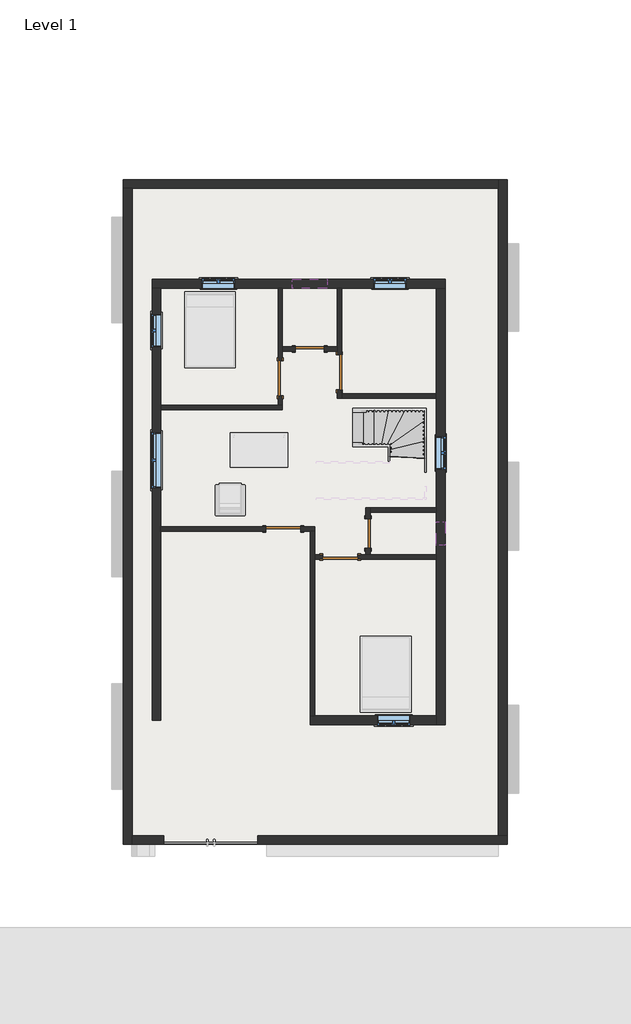
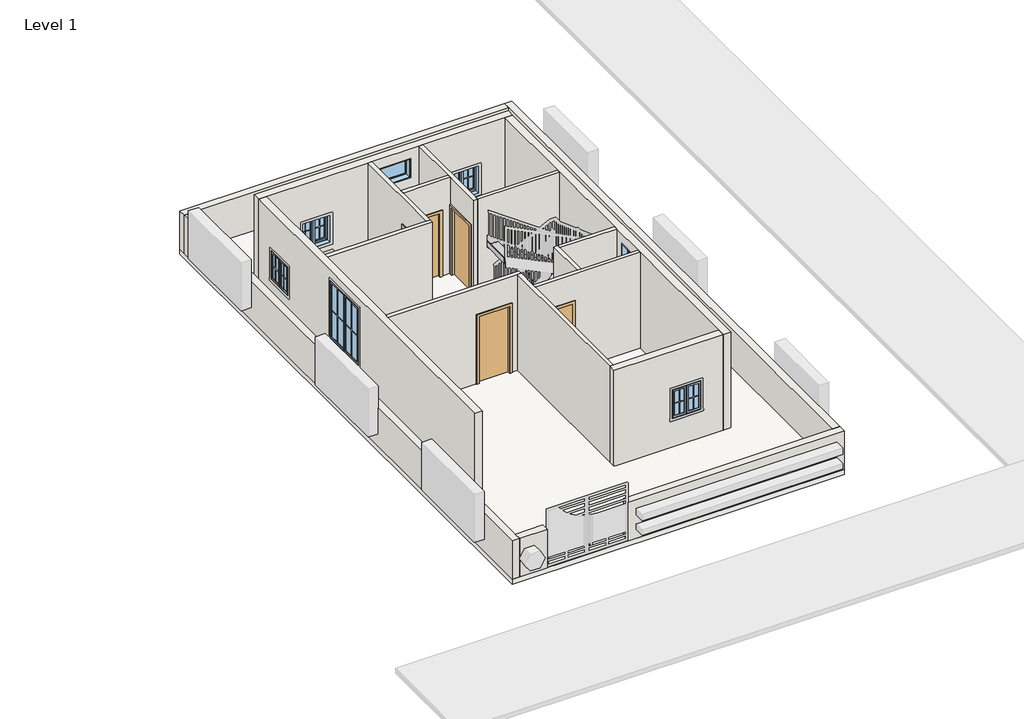
# One storey, part 1 of 3: 19 walls, 8 windows, 6 doors, 1 slab, 1 stair flight.
"""IFC4 building model written with IfcOpenShell, lengths in millimetres."""

from ifc_helpers import new_model, si_unit, frame, origin, origin_with_axes, place, context, project, spatial, polyline, outline, extrude, faceted_brep, transform, mapped, element, save
from components import door_d8f5dbb5, door_f2b275c1, door_e5f9f3c4, door_305aa2a5, stair_flight_f84afbbd, window_80340324, window_bb95b1c9, window_339605e1, window_9ac97e1a

model = new_model("IFC4")

# Units and contexts
model_context = context("Model", 3, world=origin())
ifc_project = project(units=[si_unit("LENGTHUNIT", "METRE", prefix="MILLI")], contexts=[model_context])

# Site, building, storey
site = spatial("IfcSite", under=ifc_project)
building = spatial("IfcBuilding", under=site)
storey = spatial("IfcBuildingStorey", under=building, Name="Level 1", Elevation=0.0)

# Doors
placement = place(None, origin())
door_shape = door_d8f5dbb5(model_context)
element("IfcDoor", 1, ObjectType="Single-Flush : 30\" x 80\"", at=placement, inside=storey, context=model_context, shape_type="MappedRepresentation", body=[
    mapped(door_shape, transform((-963.1415084, 4519.6435985, 0.0), x_axis=(1.0, 0.0, 0.0), y_axis=(0.0, 1.0, 0.0), z_axis=(0.0, 0.0, 1.0))),
])
door_2_shape = door_f2b275c1(model_context)
element("IfcDoor", 2, ObjectType="Single-Flush : 30\" x 80\"", at=placement, inside=storey, context=model_context, shape_type="MappedRepresentation", body=[
    mapped(door_2_shape, transform((554.5084916, -280.9564015, 0.0), x_axis=(0.0, 1.0, 0.0), y_axis=(-1.0, 0.0, 0.0), z_axis=(0.0, 0.0, 1.0))),
])
door_3_shape = door_e5f9f3c4(model_context)
element("IfcDoor", 3, ObjectType="Single-Flush : 36\" x 84\"", at=placement, inside=storey, context=model_context, shape_type="MappedRepresentation", body=[
    mapped(door_3_shape, transform((-194.7915084, 3910.0435985, 0.0), x_axis=(0.0, -1.0, 0.0), y_axis=(1.0, 0.0, 0.0), z_axis=(0.0, 0.0, 1.0))),
])
element("IfcDoor", 4, ObjectType="Single-Flush : 36\" x 84\"", at=placement, inside=storey, context=model_context, shape_type="MappedRepresentation", body=[
    mapped(door_3_shape, transform((-1655.2915084, -166.6564015, 0.0), x_axis=(1.0, 0.0, 0.0), y_axis=(0.0, 1.0, 0.0), z_axis=(0.0, 0.0, 1.0))),
])
element("IfcDoor", 5, ObjectType="Single-Flush : 36\" x 84\"", at=placement, inside=storey, context=model_context, shape_type="MappedRepresentation", body=[
    mapped(door_3_shape, transform((-169.3915084, -890.5564015, 0.0), x_axis=(-1.0, 0.0, 0.0), y_axis=(0.0, -1.0, 0.0), z_axis=(0.0, 0.0, 1.0))),
])
door_4_shape = door_305aa2a5(model_context)
element("IfcDoor", 6, ObjectType="Single-Flush : 36\" x 84\"", at=placement, inside=storey, context=model_context, shape_type="MappedRepresentation", body=[
    mapped(door_4_shape, transform((-1731.4915084, 3757.6435985, 0.0), x_axis=(0.0, -1.0, 0.0), y_axis=(1.0, 0.0, 0.0), z_axis=(0.0, 0.0, 1.0))),
])

# Slab
element("IfcSlab", 7, ObjectType="Generic - 12\"", at=placement, inside=storey, context=model_context, shape_type="SweptSolid", body=[
    extrude(outline(polyline([(4171.3077953, 8926.7169918), (4171.3077953, -8370.6830082), (-5810.8922047, -8370.6830082), (-5810.8922047, 8926.7169918), (4171.3077953, 8926.7169918)])), frame((0.0, 0.0, -152.4), z_axis=(0.0, 0.0, 1.0), x_axis=(1.0, 0.0, 0.0)), (0.0, 0.0, 1.0), 152.4),
])

# Stair flight
stair_flight_shape = stair_flight_f84afbbd(model_context)
element("IfcStairFlight", 8, ObjectType="2\" Tread 1\" Nosing 1/4\" Riser", at=placement, inside=storey, context=model_context, shape_type="MappedRepresentation", body=[
    mapped(stair_flight_shape, transform((0.0, 0.0, 0.0), x_axis=(1.0, 0.0, 0.0), y_axis=(0.0, 1.0, 0.0), z_axis=(0.0, 0.0, 1.0))),
])

# Walls
element("IfcWall", 9, ObjectType="WALL4.5\"", at=placement, inside=storey, context=model_context, shape_type="Brep", body=[
    faceted_brep([(-4836.6415084, 2938.4935985, 0.0), (-1674.3415084, 2938.4935985, 0.0), (-1674.3415084, 2938.4935985, 3048.0), (-4836.6415084, 2938.4935985, 3048.0), (-4836.6415084, 3052.7935985, 0.0), (-4836.6415084, 3052.7935985, 3048.0), (-1788.6415084, 3052.7935985, 3048.0), (-1674.3415084, 3052.7935985, 3048.0), (-1674.3415084, 3052.7935985, 0.0), (-1788.6415084, 3052.7935985, 0.0)], [[[0, 1, 2, 3]], [[4, 5, 6, 7, 8, 9]], [[1, 0, 4, 9, 8]], [[0, 3, 5, 4]], [[2, 1, 8, 7]], [[3, 2, 7, 6, 5]]]),
])
element("IfcWall", 10, ObjectType="WALL4.5\"", at=placement, inside=storey, context=model_context, shape_type="Brep", body=[
    faceted_brep([(-1674.3415084, 3052.7935985, 0.0), (-1674.3415084, 3300.4435985, 0.0), (-1674.3415084, 3300.4435985, 2133.6), (-1674.3415084, 4214.8435985, 2133.6), (-1674.3415084, 4214.8435985, 0.0), (-1674.3415084, 4462.4935985, 0.0), (-1674.3415084, 4576.7935985, 0.0), (-1674.3415084, 6100.7935985, 0.0), (-1674.3415084, 6100.7935985, 3048.0), (-1674.3415084, 4576.7935985, 3048.0), (-1674.3415084, 4462.4935985, 3048.0), (-1674.3415084, 3052.7935985, 3048.0), (-1788.6415084, 3300.4435985, 2133.6), (-1788.6415084, 3300.4435985, 0.0), (-1788.6415084, 3052.7935985, 0.0), (-1788.6415084, 3052.7935985, 3048.0), (-1788.6415084, 6100.7935985, 3048.0), (-1788.6415084, 6100.7935985, 0.0), (-1788.6415084, 4214.8435985, 0.0), (-1788.6415084, 4214.8435985, 2133.6)], [[[0, 1, 2, 3, 4, 5, 6, 7, 8, 9, 10, 11]], [[12, 13, 14, 15, 16, 17, 18, 19]], [[18, 17, 7, 6, 5, 4]], [[14, 13, 1, 0]], [[0, 11, 15, 14]], [[8, 7, 17, 16]], [[2, 1, 13, 12]], [[3, 2, 12, 19]], [[4, 3, 19, 18]], [[11, 10, 9, 8, 16, 15]]]),
])
element("IfcWall", 11, ObjectType="WALL4.5\"", at=placement, inside=storey, context=model_context, shape_type="SweptSolid", body=[
    extrude(outline(polyline([(2032.0, -582.1415084), (0.0, -582.1415084), (0.0, -251.9415084), (3048.0, -251.9415084), (3048.0, -1674.3415084), (0.0, -1674.3415084), (0.0, -1344.1415084), (2032.0, -1344.1415084), (2032.0, -582.1415084)])), frame((0.0, 4462.4935985, 0.0), z_axis=(0.0, 1.0, 0.0), x_axis=(0.0, 0.0, 1.0)), (0.0, 0.0, 1.0), 114.3),
])
element("IfcWall", 12, ObjectType="WALL4.5\"", at=placement, inside=storey, context=model_context, shape_type="Brep", body=[
    faceted_brep([(-251.9415084, 3452.8435985, 2133.6), (-251.9415084, 3452.8435985, 0.0), (-251.9415084, 3243.2935985, 0.0), (-251.9415084, 3243.2935985, 3048.0), (-251.9415084, 4462.4935985, 3048.0), (-251.9415084, 4576.7935985, 3048.0), (-251.9415084, 6100.7935985, 3048.0), (-251.9415084, 6100.7935985, 0.0), (-251.9415084, 4576.7935985, 0.0), (-251.9415084, 4462.4935985, 0.0), (-251.9415084, 4367.2435985, 0.0), (-251.9415084, 4367.2435985, 2133.6), (-137.6415084, 3243.2935985, 0.0), (-137.6415084, 3357.5935985, 0.0), (-137.6415084, 3452.8435985, 0.0), (-137.6415084, 3452.8435985, 2133.6), (-137.6415084, 4367.2435985, 2133.6), (-137.6415084, 4367.2435985, 0.0), (-137.6415084, 6100.7935985, 0.0), (-137.6415084, 6100.7935985, 3048.0), (-137.6415084, 3357.5935985, 3048.0), (-137.6415084, 3243.2935985, 3048.0)], [[[0, 1, 2, 3, 4, 5, 6, 7, 8, 9, 10, 11]], [[12, 13, 14, 15, 16, 17, 18, 19, 20, 21]], [[2, 1, 14, 13, 12]], [[10, 9, 8, 7, 18, 17]], [[7, 6, 19, 18]], [[3, 2, 12, 21]], [[15, 14, 1, 0]], [[16, 15, 0, 11]], [[17, 16, 11, 10]], [[6, 5, 4, 3, 21, 20, 19]]]),
])
element("IfcWall", 13, ObjectType="WALL4.5\"", at=placement, inside=storey, context=model_context, shape_type="SweptSolid", body=[
    extrude(outline(polyline([(2326.1584916, 3243.2935985), (-137.6415084, 3243.2935985), (-137.6415084, 3357.5935985), (2326.1584916, 3357.5935985), (2326.1584916, 3243.2935985)])), origin_with_axes(), (0.0, 0.0, 1.0), 3048.0),
])
element("IfcWall", 14, ObjectType="WALL4.5\"", at=placement, inside=storey, context=model_context, shape_type="Brep", body=[
    faceted_brep([(-1198.0915084, -223.8064015, 2133.6), (-1198.0915084, -223.8064015, 0.0), (-950.4415084, -223.8064015, 0.0), (-836.1415084, -223.8064015, 0.0), (-836.1415084, -223.8064015, 3048.0), (-950.4415084, -223.8064015, 3048.0), (-4836.6415084, -223.8064015, 3048.0), (-4836.6415084, -223.8064015, 0.0), (-2112.4915084, -223.8064015, 0.0), (-2112.4915084, -223.8064015, 2133.6), (-836.1415084, -109.5064015, 0.0), (-1198.0915084, -109.5064015, 0.0), (-1198.0915084, -109.5064015, 2133.6), (-2112.4915084, -109.5064015, 2133.6), (-2112.4915084, -109.5064015, 0.0), (-4836.6415084, -109.5064015, 0.0), (-4836.6415084, -109.5064015, 3048.0), (-836.1415084, -109.5064015, 3048.0)], [[[0, 1, 2, 3, 4, 5, 6, 7, 8, 9]], [[10, 11, 12, 13, 14, 15, 16, 17]], [[8, 7, 15, 14]], [[3, 2, 1, 11, 10]], [[7, 6, 16, 15]], [[4, 3, 10, 17]], [[12, 11, 1, 0]], [[13, 12, 0, 9]], [[14, 13, 9, 8]], [[6, 5, 4, 17, 16]]]),
])
element("IfcWall", 15, ObjectType="WALL4.5\"", at=placement, inside=storey, context=model_context, shape_type="Brep", body=[
    faceted_brep([(-950.4415084, -223.8064015, 0.0), (-950.4415084, -5024.4064015, 0.0), (-950.4415084, -5024.4064015, 3048.0), (-950.4415084, -223.8064015, 3048.0), (-836.1415084, -223.8064015, 0.0), (-836.1415084, -223.8064015, 3048.0), (-836.1415084, -833.4064015, 3048.0), (-836.1415084, -947.7064015, 3048.0), (-836.1415084, -5024.4064015, 3048.0), (-836.1415084, -5024.4064015, 0.0), (-836.1415084, -947.7064015, 0.0), (-836.1415084, -833.4064015, 0.0)], [[[0, 1, 2, 3]], [[4, 5, 6, 7, 8, 9, 10, 11]], [[2, 1, 9, 8]], [[0, 3, 5, 4]], [[1, 0, 4, 11, 10, 9]], [[3, 2, 8, 7, 6, 5]]]),
])
element("IfcWall", 16, ObjectType="WALL4.5\"", at=placement, inside=storey, context=model_context, shape_type="Brep", body=[
    faceted_brep([(-836.1415084, -947.7064015, 0.0), (-626.5915084, -947.7064015, 0.0), (-626.5915084, -947.7064015, 2133.6), (287.8084916, -947.7064015, 2133.6), (287.8084916, -947.7064015, 0.0), (2326.1584916, -947.7064015, 0.0), (2326.1584916, -947.7064015, 3048.0), (-836.1415084, -947.7064015, 3048.0), (-626.5915084, -833.4064015, 2133.6), (-626.5915084, -833.4064015, 0.0), (-836.1415084, -833.4064015, 0.0), (-836.1415084, -833.4064015, 3048.0), (497.3584916, -833.4064015, 3048.0), (611.6584916, -833.4064015, 3048.0), (2326.1584916, -833.4064015, 3048.0), (2326.1584916, -833.4064015, 0.0), (611.6584916, -833.4064015, 0.0), (497.3584916, -833.4064015, 0.0), (287.8084916, -833.4064015, 0.0), (287.8084916, -833.4064015, 2133.6)], [[[0, 1, 2, 3, 4, 5, 6, 7]], [[8, 9, 10, 11, 12, 13, 14, 15, 16, 17, 18, 19]], [[10, 9, 1, 0]], [[18, 17, 16, 15, 5, 4]], [[6, 5, 15, 14]], [[0, 7, 11, 10]], [[2, 1, 9, 8]], [[3, 2, 8, 19]], [[4, 3, 19, 18]], [[7, 6, 14, 13, 12, 11]]]),
])
element("IfcWall", 17, ObjectType="WALL4.5\"", at=placement, inside=storey, context=model_context, shape_type="Brep", body=[
    faceted_brep([(611.6584916, 100.0435985, 2032.0), (611.6584916, 100.0435985, 0.0), (611.6584916, 271.4935985, 0.0), (611.6584916, 385.7935985, 0.0), (611.6584916, 385.7935985, 3048.0), (611.6584916, 271.4935985, 3048.0), (611.6584916, -833.4064015, 3048.0), (611.6584916, -833.4064015, 0.0), (611.6584916, -661.9564015, 0.0), (611.6584916, -661.9564015, 2032.0), (497.3584916, 385.7935985, 0.0), (497.3584916, 100.0435985, 0.0), (497.3584916, 100.0435985, 2032.0), (497.3584916, -661.9564015, 2032.0), (497.3584916, -661.9564015, 0.0), (497.3584916, -833.4064015, 0.0), (497.3584916, -833.4064015, 3048.0), (497.3584916, 385.7935985, 3048.0)], [[[0, 1, 2, 3, 4, 5, 6, 7, 8, 9]], [[10, 11, 12, 13, 14, 15, 16, 17]], [[8, 7, 15, 14]], [[3, 2, 1, 11, 10]], [[7, 6, 16, 15]], [[4, 3, 10, 17]], [[12, 11, 1, 0]], [[13, 12, 0, 9]], [[14, 13, 9, 8]], [[6, 5, 4, 17, 16]]]),
])
element("IfcWall", 18, ObjectType="WALL4.5\"", at=placement, inside=storey, context=model_context, shape_type="SweptSolid", body=[
    extrude(outline(polyline([(2326.1584916, 271.4935985), (611.6584916, 271.4935985), (611.6584916, 385.7935985), (2326.1584916, 385.7935985), (2326.1584916, 271.4935985)])), origin_with_axes(), (0.0, 0.0, 1.0), 3048.0),
])
element("IfcWall", 19, ObjectType="WALL9\"", at=placement, inside=storey, context=model_context, shape_type="Brep", body=[
    faceted_brep([(-5065.2415084, 6100.7935985, 0.0), (-4836.6415084, 6100.7935985, 0.0), (-1788.6415084, 6100.7935985, 0.0), (-1674.3415084, 6100.7935985, 0.0), (-251.9415084, 6100.7935985, 0.0), (-137.6415084, 6100.7935985, 0.0), (2326.1584916, 6100.7935985, 0.0), (2554.7584916, 6100.7935985, 0.0), (2554.7584916, 6100.7935985, 3048.0), (2326.1584916, 6100.7935985, 3048.0), (-137.6415084, 6100.7935985, 3048.0), (-251.9415084, 6100.7935985, 3048.0), (-1674.3415084, 6100.7935985, 3048.0), (-1788.6415084, 6100.7935985, 3048.0), (-4836.6415084, 6100.7935985, 3048.0), (-5065.2415084, 6100.7935985, 3048.0), (-505.9415084, 6100.7935985, 2743.2), (-505.9415084, 6100.7935985, 2133.6), (-1420.3415084, 6100.7935985, 2133.6), (-1420.3415084, 6100.7935985, 2743.2), (-2909.4165084, 6100.7935985, 1828.8), (-2909.4165084, 6100.7935985, 914.4), (-3773.0165084, 6100.7935985, 914.4), (-3773.0165084, 6100.7935985, 1828.8), (1554.6334916, 6100.7935985, 1828.8), (1554.6334916, 6100.7935985, 914.4), (691.0334916, 6100.7935985, 914.4), (691.0334916, 6100.7935985, 1828.8), (-5065.2415084, 6329.3935985, 0.0), (-5065.2415084, 6329.3935985, 3048.0), (2554.7584916, 6329.3935985, 3048.0), (2554.7584916, 6329.3935985, 0.0), (-505.9415084, 6329.3935985, 2743.2), (-1420.3415084, 6329.3935985, 2743.2), (-1420.3415084, 6329.3935985, 2133.6), (-505.9415084, 6329.3935985, 2133.6), (-2909.4165084, 6329.3935985, 1828.8), (-3773.0165084, 6329.3935985, 1828.8), (-3773.0165084, 6329.3935985, 914.4), (-2909.4165084, 6329.3935985, 914.4), (1554.6334916, 6329.3935985, 1828.8), (691.0334916, 6329.3935985, 1828.8), (691.0334916, 6329.3935985, 914.4), (1554.6334916, 6329.3935985, 914.4)], [[[0, 1, 2, 3, 4, 5, 6, 7, 8, 9, 10, 11, 12, 13, 14, 15], [16, 17, 18, 19], [20, 21, 22, 23], [24, 25, 26, 27]], [[28, 29, 30, 31], [32, 33, 34, 35], [36, 37, 38, 39], [40, 41, 42, 43]], [[7, 6, 5, 4, 3, 2, 1, 0, 28, 31]], [[8, 7, 31, 30]], [[0, 15, 29, 28]], [[17, 16, 32, 35]], [[18, 17, 35, 34]], [[19, 18, 34, 33]], [[16, 19, 33, 32]], [[21, 20, 36, 39]], [[22, 21, 39, 38]], [[23, 22, 38, 37]], [[20, 23, 37, 36]], [[25, 24, 40, 43]], [[26, 25, 43, 42]], [[27, 26, 42, 41]], [[24, 27, 41, 40]], [[15, 14, 13, 12, 11, 10, 9, 8, 30, 29]]]),
])
element("IfcWall", 20, ObjectType="WALL9\"", at=placement, inside=storey, context=model_context, shape_type="Brep", body=[
    faceted_brep([(2326.1584916, 6100.7935985, 0.0), (2326.1584916, 3357.5935985, 0.0), (2326.1584916, 3243.2935985, 0.0), (2326.1584916, 385.7935985, 0.0), (2326.1584916, 271.4935985, 0.0), (2326.1584916, -833.4064015, 0.0), (2326.1584916, -947.7064015, 0.0), (2326.1584916, -5024.4064015, 0.0), (2326.1584916, -5253.0064015, 0.0), (2326.1584916, -5253.0064015, 3048.0), (2326.1584916, -5024.4064015, 3048.0), (2326.1584916, -947.7064015, 3048.0), (2326.1584916, -833.4064015, 3048.0), (2326.1584916, 271.4935985, 3048.0), (2326.1584916, 385.7935985, 3048.0), (2326.1584916, 3243.2935985, 3048.0), (2326.1584916, 3357.5935985, 3048.0), (2326.1584916, 6100.7935985, 3048.0), (2326.1584916, -585.7564015, 2743.2), (2326.1584916, -585.7564015, 2133.6), (2326.1584916, 23.8435985, 2133.6), (2326.1584916, 23.8435985, 2743.2), (2326.1584916, 1382.7435985, 1828.8), (2326.1584916, 1382.7435985, 914.4), (2326.1584916, 2246.3435985, 914.4), (2326.1584916, 2246.3435985, 1828.8), (2554.7584916, 6100.7935985, 0.0), (2554.7584916, 6100.7935985, 3048.0), (2554.7584916, -5253.0064015, 3048.0), (2554.7584916, -5253.0064015, 0.0), (2554.7584916, -585.7564015, 2743.2), (2554.7584916, 23.8435985, 2743.2), (2554.7584916, 23.8435985, 2133.6), (2554.7584916, -585.7564015, 2133.6), (2554.7584916, 1382.7435985, 1828.8), (2554.7584916, 2246.3435985, 1828.8), (2554.7584916, 2246.3435985, 914.4), (2554.7584916, 1382.7435985, 914.4)], [[[0, 1, 2, 3, 4, 5, 6, 7, 8, 9, 10, 11, 12, 13, 14, 15, 16, 17], [18, 19, 20, 21], [22, 23, 24, 25]], [[26, 27, 28, 29], [30, 31, 32, 33], [34, 35, 36, 37]], [[8, 7, 6, 5, 4, 3, 2, 1, 0, 26, 29]], [[0, 17, 27, 26]], [[9, 8, 29, 28]], [[19, 18, 30, 33]], [[20, 19, 33, 32]], [[21, 20, 32, 31]], [[18, 21, 31, 30]], [[23, 22, 34, 37]], [[24, 23, 37, 36]], [[25, 24, 36, 35]], [[22, 25, 35, 34]], [[17, 16, 15, 14, 13, 12, 11, 10, 9, 28, 27]]]),
])
element("IfcWall", 21, ObjectType="WALL9\"", at=placement, inside=storey, context=model_context, shape_type="Brep", body=[
    faceted_brep([(2326.1584916, -5024.4064015, 0.0), (-836.1415084, -5024.4064015, 0.0), (-950.4415084, -5024.4064015, 0.0), (-950.4415084, -5024.4064015, 3048.0), (-836.1415084, -5024.4064015, 3048.0), (2326.1584916, -5024.4064015, 3048.0), (789.4584916, -5024.4064015, 1828.8), (789.4584916, -5024.4064015, 914.4), (1653.0584916, -5024.4064015, 914.4), (1653.0584916, -5024.4064015, 1828.8), (2326.1584916, -5253.0064015, 0.0), (2326.1584916, -5253.0064015, 3048.0), (-950.4415084, -5253.0064015, 3048.0), (-950.4415084, -5253.0064015, 0.0), (789.4584916, -5253.0064015, 1828.8), (1653.0584916, -5253.0064015, 1828.8), (1653.0584916, -5253.0064015, 914.4), (789.4584916, -5253.0064015, 914.4)], [[[0, 1, 2, 3, 4, 5], [6, 7, 8, 9]], [[10, 11, 12, 13], [14, 15, 16, 17]], [[2, 1, 0, 10, 13]], [[0, 5, 11, 10]], [[3, 2, 13, 12]], [[7, 6, 14, 17]], [[8, 7, 17, 16]], [[9, 8, 16, 15]], [[6, 9, 15, 14]], [[5, 4, 3, 12, 11]]]),
])
element("IfcWall", 22, ObjectType="WALL9\"", at=placement, inside=storey, context=model_context, shape_type="Brep", body=[
    faceted_brep([(-5065.2415084, 6100.7935985, 0.0), (-5065.2415084, -5138.7064015, 0.0), (-5065.2415084, -5138.7064015, 3048.0), (-5065.2415084, 6100.7935985, 3048.0), (-5065.2415084, 2347.9435985, 2743.2), (-5065.2415084, 900.1435985, 2743.2), (-5065.2415084, 900.1435985, 914.4), (-5065.2415084, 2347.9435985, 914.4), (-5065.2415084, 5427.6935985, 1828.8), (-5065.2415084, 4564.0935985, 1828.8), (-5065.2415084, 4564.0935985, 914.4), (-5065.2415084, 5427.6935985, 914.4), (-4836.6415084, 6100.7935985, 0.0), (-4836.6415084, 6100.7935985, 3048.0), (-4836.6415084, 3052.7935985, 3048.0), (-4836.6415084, 2938.4935985, 3048.0), (-4836.6415084, -109.5064015, 3048.0), (-4836.6415084, -223.8064015, 3048.0), (-4836.6415084, -5138.7064015, 3048.0), (-4836.6415084, -5138.7064015, 0.0), (-4836.6415084, -223.8064015, 0.0), (-4836.6415084, -109.5064015, 0.0), (-4836.6415084, 2938.4935985, 0.0), (-4836.6415084, 3052.7935985, 0.0), (-4836.6415084, 2347.9435985, 2743.2), (-4836.6415084, 2347.9435985, 914.4), (-4836.6415084, 900.1435985, 914.4), (-4836.6415084, 900.1435985, 2743.2), (-4836.6415084, 5427.6935985, 1828.8), (-4836.6415084, 5427.6935985, 914.4), (-4836.6415084, 4564.0935985, 914.4), (-4836.6415084, 4564.0935985, 1828.8)], [[[0, 1, 2, 3], [4, 5, 6, 7], [8, 9, 10, 11]], [[12, 13, 14, 15, 16, 17, 18, 19, 20, 21, 22, 23], [24, 25, 26, 27], [28, 29, 30, 31]], [[1, 0, 12, 23, 22, 21, 20, 19]], [[2, 1, 19, 18]], [[0, 3, 13, 12]], [[25, 24, 4, 7]], [[26, 25, 7, 6]], [[27, 26, 6, 5]], [[24, 27, 5, 4]], [[29, 28, 8, 11]], [[30, 29, 11, 10]], [[31, 30, 10, 9]], [[28, 31, 9, 8]], [[3, 2, 18, 17, 16, 15, 14, 13]]]),
])
element("IfcWall", 23, ObjectType="WALL9\"", at=placement, inside=storey, context=model_context, shape_type="Brep", body=[
    faceted_brep([(-5810.8922047, 8698.1169918, 0.0), (-5582.2922047, 8698.1169918, 0.0), (3942.7077953, 8698.1169918, 0.0), (3942.7077953, 8698.1169918, 1219.2), (-5582.2922047, 8698.1169918, 1219.2), (-5810.8922047, 8698.1169918, 1219.2), (-5810.8922047, 8926.7169918, 0.0), (-5810.8922047, 8926.7169918, 1219.2), (3942.7077953, 8926.7169918, 1219.2), (3942.7077953, 8926.7169918, 0.0)], [[[0, 1, 2, 3, 4, 5]], [[6, 7, 8, 9]], [[2, 1, 0, 6, 9]], [[5, 4, 3, 8, 7]], [[0, 5, 7, 6]], [[3, 2, 9, 8]]]),
])
element("IfcWall", 24, ObjectType="WALL9\"", at=placement, inside=storey, context=model_context, shape_type="Brep", body=[
    faceted_brep([(-5582.2922047, -8370.6830082, 0.0), (-5582.2922047, -8142.0830082, 0.0), (-5582.2922047, 8698.1169918, 0.0), (-5582.2922047, 8698.1169918, 1219.2), (-5582.2922047, -8142.0830082, 1219.2), (-5582.2922047, -8370.6830082, 1219.2), (-5810.8922047, -8370.6830082, 0.0), (-5810.8922047, -8370.6830082, 1219.2), (-5810.8922047, 8698.1169918, 1219.2), (-5810.8922047, 8698.1169918, 0.0)], [[[0, 1, 2, 3, 4, 5]], [[6, 7, 8, 9]], [[2, 1, 0, 6, 9]], [[5, 4, 3, 8, 7]], [[0, 5, 7, 6]], [[3, 2, 9, 8]]]),
])
element("IfcWall", 25, ObjectType="WALL9\"", at=placement, inside=storey, context=model_context, shape_type="Brep", body=[
    faceted_brep([(4171.3077953, -8142.0830082, 0.0), (3942.7077953, -8142.0830082, 0.0), (-2318.3922047, -8142.0830082, 0.0), (-2318.3922047, -8142.0830082, 1219.2), (3942.7077953, -8142.0830082, 1219.2), (4171.3077953, -8142.0830082, 1219.2), (4171.3077953, -8370.6830082, 0.0), (4171.3077953, -8370.6830082, 1219.2), (-2318.3922047, -8370.6830082, 1219.2), (-2318.3922047, -8370.6830082, 0.0)], [[[0, 1, 2, 3, 4, 5]], [[6, 7, 8, 9]], [[2, 1, 0, 6, 9]], [[3, 2, 9, 8]], [[5, 4, 3, 8, 7]], [[0, 5, 7, 6]]]),
])
element("IfcWall", 26, ObjectType="WALL9\"", at=placement, inside=storey, context=model_context, shape_type="Brep", body=[
    faceted_brep([(3942.7077953, 8926.7169918, 0.0), (3942.7077953, 8698.1169918, 0.0), (3942.7077953, -8142.0830082, 0.0), (3942.7077953, -8142.0830082, 1219.2), (3942.7077953, 8698.1169918, 1219.2), (3942.7077953, 8926.7169918, 1219.2), (4171.3077953, 8926.7169918, 0.0), (4171.3077953, 8926.7169918, 1219.2), (4171.3077953, -8142.0830082, 1219.2), (4171.3077953, -8142.0830082, 0.0)], [[[0, 1, 2, 3, 4, 5]], [[6, 7, 8, 9]], [[2, 1, 0, 6, 9]], [[5, 4, 3, 8, 7]], [[0, 5, 7, 6]], [[3, 2, 9, 8]]]),
])
element("IfcWall", 27, ObjectType="WALL9\"", at=placement, inside=storey, context=model_context, shape_type="SweptSolid", body=[
    extrude(outline(polyline([(-5582.2922047, -8142.0830082), (-4756.7922047, -8142.0830082), (-4756.7922047, -8370.6830082), (-5582.2922047, -8370.6830082), (-5582.2922047, -8142.0830082)])), origin_with_axes(), (0.0, 0.0, 1.0), 1219.2),
])

# Windows
window_shape = window_80340324(model_context)
element("IfcWindow", 28, ObjectType="Fixed : 24\" x 24\"", at=placement, inside=storey, context=model_context, shape_type="MappedRepresentation", body=[
    mapped(window_shape, transform((2440.4584916, -319.0564015, 1219.2), x_axis=(0.0, -1.0, 0.0), y_axis=(1.0, 0.0, 0.0), z_axis=(0.0, 0.0, 1.0))),
])
window_2_shape = window_bb95b1c9(model_context)
element("IfcWindow", 29, ObjectType="Fixed : 36\" x 24\"", at=placement, inside=storey, context=model_context, shape_type="MappedRepresentation", body=[
    mapped(window_2_shape, transform((-925.0415084, 6215.0935985, 1219.2), x_axis=(1.0, 0.0, 0.0), y_axis=(0.0, 1.0, 0.0), z_axis=(0.0, 0.0, 1.0))),
])
window_3_shape = window_339605e1(model_context)
element("IfcWindow", 30, ObjectType="Window-Casement-Double : 34\" x 36\"", at=placement, inside=storey, context=model_context, shape_type="MappedRepresentation", body=[
    mapped(window_3_shape, transform((-3341.2165084, 6215.0935985, 0.0), x_axis=(1.0, 0.0, 0.0), y_axis=(0.0, 1.0, 0.0), z_axis=(0.0, 0.0, 1.0))),
])
element("IfcWindow", 31, ObjectType="Window-Casement-Double : 34\" x 36\"", at=placement, inside=storey, context=model_context, shape_type="MappedRepresentation", body=[
    mapped(window_3_shape, transform((1221.2584916, -5138.7064015, 0.0), x_axis=(-1.0, 0.0, 0.0), y_axis=(0.0, -1.0, 0.0), z_axis=(0.0, 0.0, 1.0))),
])
element("IfcWindow", 32, ObjectType="Window-Casement-Double : 34\" x 36\"", at=placement, inside=storey, context=model_context, shape_type="MappedRepresentation", body=[
    mapped(window_3_shape, transform((2440.4584916, 1814.5435985, 0.0), x_axis=(0.0, -1.0, 0.0), y_axis=(1.0, 0.0, 0.0), z_axis=(0.0, 0.0, 1.0))),
])
element("IfcWindow", 33, ObjectType="Window-Casement-Double : 34\" x 36\"", at=placement, inside=storey, context=model_context, shape_type="MappedRepresentation", body=[
    mapped(window_3_shape, transform((1122.8334916, 6215.0935985, 0.0), x_axis=(1.0, 0.0, 0.0), y_axis=(0.0, 1.0, 0.0), z_axis=(0.0, 0.0, 1.0))),
])
element("IfcWindow", 34, ObjectType="Window-Casement-Double : 34\" x 36\"", at=placement, inside=storey, context=model_context, shape_type="MappedRepresentation", body=[
    mapped(window_3_shape, transform((-4950.9415084, 4995.8935985, 0.0), x_axis=(0.0, 1.0, 0.0), y_axis=(-1.0, 0.0, 0.0), z_axis=(0.0, 0.0, 1.0))),
])
window_4_shape = window_9ac97e1a(model_context)
element("IfcWindow", 35, ObjectType="Window-Casement-Double : 57\" x 72\"", at=placement, inside=storey, context=model_context, shape_type="MappedRepresentation", body=[
    mapped(window_4_shape, transform((-4950.9415084, 1624.0435985, 0.0), x_axis=(0.0, 1.0, 0.0), y_axis=(-1.0, 0.0, 0.0), z_axis=(0.0, 0.0, 1.0))),
])

save(model, "model.ifc")

# Revit data of these elements
# Type "Single-Flush : 30\" x 80\""
#   Type Mark = "5"
#   Construction Type Id = "MDOOR"
#   Assembly Code = "C1020"
#   Analytic Construction = "Metal"
#   Thickness = 0' - 2"
#   Heat Transfer Coefficient (U) = 0.651978 BTU/(h·ft²·°F)
#   Height = 6' - 8"
#   Trim Projection Ext = 0' - 1"
#   Trim Projection Int = 0' - 1"
#   Trim Width = 0' - 3"
#   Width = 2' - 6"
#   Define Thermal Properties by = 1
#   Define Thermal Properties by = 1
#   Door Material = Door - Panel
#   Frame Material = Door - Frame
#   Visual Light Transmittance = 0
#   Solar Heat Gain Coefficient = 0
#   Function = (empty or 0)
#   Wall Closure = (empty or 0)
# Type "Single-Flush : 36\" x 84\""
#   Type Mark = "1"
#   Construction Type Id = "MDOOR"
#   Assembly Code = "C1020"
#   Analytic Construction = "Metal"
#   Thickness = 0' - 2"
#   Heat Transfer Coefficient (U) = 0.651978 BTU/(h·ft²·°F)
#   Height = 7' - 0"
#   Trim Projection Ext = 0' - 1"
#   Trim Projection Int = 0' - 1"
#   Trim Width = 0' - 3"
#   Width = 3' - 0"
#   Define Thermal Properties by = 1
#   Define Thermal Properties by = 1
#   Door Material = Door - Panel
#   Frame Material = Door - Frame
#   Visual Light Transmittance = 0
#   Solar Heat Gain Coefficient = 0
#   Function = (empty or 0)
#   Wall Closure = (empty or 0)
# Type "Generic - 12\""
#   Assembly Code = "B1010"
#   Function = 0
#   Layers, outside or top first: 0' - 6" no material (function 1)
# Type "WALL4.5\""
#   Assembly Code = "B2010"
#   Layers, outside or top first: 0' - 4 1/2" no material (function 1)
# Type "WALL9\""
#   Assembly Code = "B2010"
#   Layers, outside or top first: 0' - 9" no material (function 1)
# Type "Fixed : 24\" x 24\""
#   Type Mark = "3"
#   Construction Type Id = "GSP4R"
#   Assembly Code = "B2020100"
#   Analytic Construction = "1/8 in Pilkington single glazing"
#   Visual Light Transmittance = 0.9
#   Solar Heat Gain Coefficient = 0.78
#   Heat Transfer Coefficient (U) = 0.6496 BTU/(h·ft²·°F)
#   Height = 2' - 0"
#   Default Sill Height = 3' - 0"
#   Width = 2' - 0"
#   Window Inset = 0' - 0 3/4"
#   Define Thermal Properties by = 1
#   Define Thermal Properties by = 1
#   Glass Pane Material = Glass
#   Sash Material = Sash
#   Wall Closure = (empty or 0)
# Type "Fixed : 36\" x 24\""
#   Type Mark = "8"
#   Construction Type Id = "GSP4R"
#   Assembly Code = "B2020100"
#   Analytic Construction = "1/8 in Pilkington single glazing"
#   Visual Light Transmittance = 0.9
#   Solar Heat Gain Coefficient = 0.78
#   Heat Transfer Coefficient (U) = 0.6496 BTU/(h·ft²·°F)
#   Height = 2' - 0"
#   Default Sill Height = 3' - 0"
#   Width = 3' - 0"
#   Window Inset = 0' - 0 3/4"
#   Define Thermal Properties by = 1
#   Define Thermal Properties by = 1
#   Glass Pane Material = Glass
#   Sash Material = Sash
#   Wall Closure = (empty or 0)
# Type "Window-Casement-Double : 34\" x 36\""
#   Type Mark = "14"
#   Fire Rating = "0.5h"
#   Assembly Code = "B2020100"
#   Analytic Construction = "Double glazing - domestic"
#   Frame Extension [instance default] = 0' - 0 1/4"
#   Window Inset [instance default] = 0' - 0"
#   Wall Thickness [instance default] = 0' - 6"
#   Interior Wall Closure [instance default] = 0' - 2 1/4"
#   Half Width = 1' - 5"
#   Visual Light Transmittance = 0.81
#   Thermal Resistance (R) = 1.8146 (h·ft²·°F)/BTU
#   Solar Heat Gain Coefficient = 0.76
#   Rough Width = 2' - 10 1/2"
#   Rough Height = 3' - 0 1/2"
#   Height = 3' - 0"
#   Heat Transfer Coefficient (U) = 0.5511 BTU/(h·ft²·°F)
#   Exterior Wall Closure [instance default] = 0' - 1 1/4"
#   Extension Jamb [instance default] = 0' - 2 1/4"
#   Default Sill Height = 3' - 0"
#   Width = 2' - 10"
#   Define Thermal Properties by = 0
#   Muntin Visibility = yes
#   Interior Trim Visibility [instance default] = yes
#   Exterior Trim Visibility [instance default] = yes
#   Extension Jamb Visibility [instance default] = yes
#   Interior Trim Material = Wood - Stained
#   Muntin Pattern = Muntin Pattern_2x2 : Muntin Pattern_2x2
#   Interior Trim = Trim-Window-Interior-Flat : Picture Frame
#   Interior Frame Material = Wood - Stained
#   Glass Panel Material = Glass
#   Exterior Trim Material = Clad - White
#   Exterior Trim = Trim-Window-Exterior-Flat : with Sill
#   Exterior Frame Material = Clad - White
#   Wall Closure = (empty or 0)
# Type "Window-Casement-Double : 57\" x 72\""
#   Type Mark = "17"
#   Fire Rating = "0.5h"
#   Assembly Code = "B2020100"
#   Analytic Construction = "Double glazing - domestic"
#   Frame Extension [instance default] = 0' - 0 1/4"
#   Window Inset [instance default] = 0' - 0"
#   Wall Thickness [instance default] = 0' - 6"
#   Interior Wall Closure [instance default] = 0' - 2 1/4"
#   Half Width = 2' - 4 1/2"
#   Visual Light Transmittance = 0.81
#   Thermal Resistance (R) = 1.8146 (h·ft²·°F)/BTU
#   Solar Heat Gain Coefficient = 0.76
#   Rough Width = 4' - 9 1/2"
#   Rough Height = 6' - 0 1/2"
#   Height = 6' - 0"
#   Heat Transfer Coefficient (U) = 0.5511 BTU/(h·ft²·°F)
#   Exterior Wall Closure [instance default] = 0' - 1 1/4"
#   Extension Jamb [instance default] = 0' - 2 1/4"
#   Default Sill Height = 3' - 0"
#   Width = 4' - 9"
#   Define Thermal Properties by = 0
#   Muntin Visibility = yes
#   Interior Trim Visibility [instance default] = yes
#   Exterior Trim Visibility [instance default] = yes
#   Extension Jamb Visibility [instance default] = yes
#   Interior Trim Material = Wood - Stained
#   Muntin Pattern = Muntin Pattern_2x2 : Muntin Pattern_2x2
#   Interior Trim = Trim-Window-Interior-Flat : Picture Frame
#   Interior Frame Material = Wood - Stained
#   Glass Panel Material = Glass
#   Exterior Trim Material = Clad - White
#   Exterior Trim = Trim-Window-Exterior-Flat : with Sill
#   Exterior Frame Material = Clad - White
#   Wall Closure = (empty or 0)
# Elements 1, 2 (IfcDoor, "Single-Flush : 30\" x 80\"")
#   Phase Created = New Construction
#   Materials on its faces: "Door - Frame", "Door - Panel"
# Elements 3, 4, 5, 6 (IfcDoor, "Single-Flush : 36\" x 84\"")
#   Phase Created = New Construction
#   Materials on its faces: "Door - Frame", "Door - Panel"
# Element 7 (IfcSlab, "Generic - 12\"")
#   Height Offset From Level = 0' - 0"
#   Phase Created = New Construction
#   Materials on its faces: "Default Floor"
# Element 8 (IfcStairFlight, "2\" Tread 1\" Nosing 1/4\" Riser")
#   Phase Created = New Construction
# Elements 9, 10, 11, 12, 13, 15, 16, 17, 18 (IfcWall, "WALL4.5\"")
#   Top Offset = 0' - 0"
#   Base Offset = 0' - 0"
#   Unconnected Height = 10' - 0"
#   wall height = 10' - 0"
#   Phase Created = New Construction
#   Base Constraint = Level 1
#   Materials on its faces: "Default Wall"
# Element 14 (IfcWall, "WALL4.5\"")
#   Top Offset = 0' - 0"
#   Base Offset = 0' - 0"
#   Unconnected Height = 10' - 0"
#   wall height = 10' - 0"
#   Phase Created = New Construction
#   Base Constraint = Level 1
#   Materials on its faces: "Default Wall", "Plywood, Sheathing"
# Elements 19, 20, 21, 22 (IfcWall, "WALL9\"")
#   Top Offset = 0' - 0"
#   Base Offset = 0' - 0"
#   Unconnected Height = 10' - 0"
#   wall height = 10' - 0"
#   Phase Created = New Construction
#   Base Constraint = Level 1
#   Materials on its faces: "Default Wall", "Plywood, Sheathing"
# Elements 23, 24, 25, 26, 27 (IfcWall, "WALL9\"")
#   Top Offset = 0' - 0"
#   Base Offset = 0' - 0"
#   Unconnected Height = 4' - 0"
#   wall height = 4' - 0"
#   Phase Created = New Construction
#   Base Constraint = Level 1
#   Materials on its faces: "Default Wall"
# Element 28 (IfcWindow, "Fixed : 24\" x 24\"")
#   Mark = "2"
#   Phase Created = New Construction
#   Materials on its faces: "Sash", "Glass"
# Element 29 (IfcWindow, "Fixed : 36\" x 24\"")
#   Mark = "1"
#   Phase Created = New Construction
#   Materials on its faces: "Sash", "Glass"
# Element 30 (IfcWindow, "Window-Casement-Double : 34\" x 36\"")
#   Mark = "3"
#   Window Inset = 0' - 0"
#   Interior Wall Closure = 0' - 2 1/4"
#   Frame Extension = 0' - 0 1/4"
#   Exterior Wall Closure = 0' - 1 1/4"
#   Interior Trim Visibility = yes
#   Exterior Trim Visibility = yes
#   Phase Created = New Construction
#   Materials on its faces: "Wood - Stained", "Glass", "Clad - White"
# Element 31 (IfcWindow, "Window-Casement-Double : 34\" x 36\"")
#   Mark = "4"
#   Window Inset = 0' - 0"
#   Interior Wall Closure = 0' - 2 1/4"
#   Frame Extension = 0' - 0 1/4"
#   Exterior Wall Closure = 0' - 1 1/4"
#   Interior Trim Visibility = yes
#   Exterior Trim Visibility = yes
#   Phase Created = New Construction
#   Materials on its faces: "Wood - Stained", "Glass", "Clad - White"
# Element 32 (IfcWindow, "Window-Casement-Double : 34\" x 36\"")
#   Mark = "6"
#   Window Inset = 0' - 0"
#   Interior Wall Closure = 0' - 2 1/4"
#   Frame Extension = 0' - 0 1/4"
#   Exterior Wall Closure = 0' - 1 1/4"
#   Interior Trim Visibility = yes
#   Exterior Trim Visibility = yes
#   Phase Created = New Construction
#   Materials on its faces: "Wood - Stained", "Glass", "Clad - White"
# Element 33 (IfcWindow, "Window-Casement-Double : 34\" x 36\"")
#   Mark = "7"
#   Window Inset = 0' - 0"
#   Interior Wall Closure = 0' - 2 1/4"
#   Frame Extension = 0' - 0 1/4"
#   Exterior Wall Closure = 0' - 1 1/4"
#   Interior Trim Visibility = yes
#   Exterior Trim Visibility = yes
#   Phase Created = New Construction
#   Materials on its faces: "Wood - Stained", "Glass", "Clad - White"
# Element 34 (IfcWindow, "Window-Casement-Double : 34\" x 36\"")
#   Mark = "8"
#   Window Inset = 0' - 0"
#   Interior Wall Closure = 0' - 2 1/4"
#   Frame Extension = 0' - 0 1/4"
#   Exterior Wall Closure = 0' - 1 1/4"
#   Interior Trim Visibility = yes
#   Exterior Trim Visibility = yes
#   Phase Created = New Construction
#   Materials on its faces: "Wood - Stained", "Glass", "Clad - White"
# Element 35 (IfcWindow, "Window-Casement-Double : 57\" x 72\"")
#   Mark = "5"
#   Window Inset = 0' - 0"
#   Interior Wall Closure = 0' - 2 1/4"
#   Frame Extension = 0' - 0 1/4"
#   Exterior Wall Closure = 0' - 1 1/4"
#   Interior Trim Visibility = yes
#   Exterior Trim Visibility = yes
#   Phase Created = New Construction
#   Materials on its faces: "Wood - Stained", "Glass", "Clad - White"
# Materials
#   "Door - Panel": class "Wood", colour RGB 210 159 95, transparency 0, Cost = 0
#   "Door - Frame": colour RGB 118 70 51, transparency 0, Cost = 0
#   "Glass": class "Glass", colour RGB 0 128 192, transparency 0.75, Description = "Soda Lime Glass", Cost = 0
#   "Sash": class "Wood", colour RGB 224 178 126, transparency 0, Cost = 0
#   "Wood - Stained": class "Wood", colour RGB 224 178 126, transparency 0, Cost = 0
#   "Clad - White": class "Wood", colour RGB 242 242 238, transparency 0, Cost = 0
#   "Default Floor": colour RGB 128 128 128, transparency 0, Cost = 0
#   "Default Wall": colour RGB 128 128 128, transparency 0, Cost = 0
#   "Plywood, Sheathing": class "Wood", colour RGB 212 179 113, transparency 0, Description = "Plywood, sheathing grade", Cost = 0
